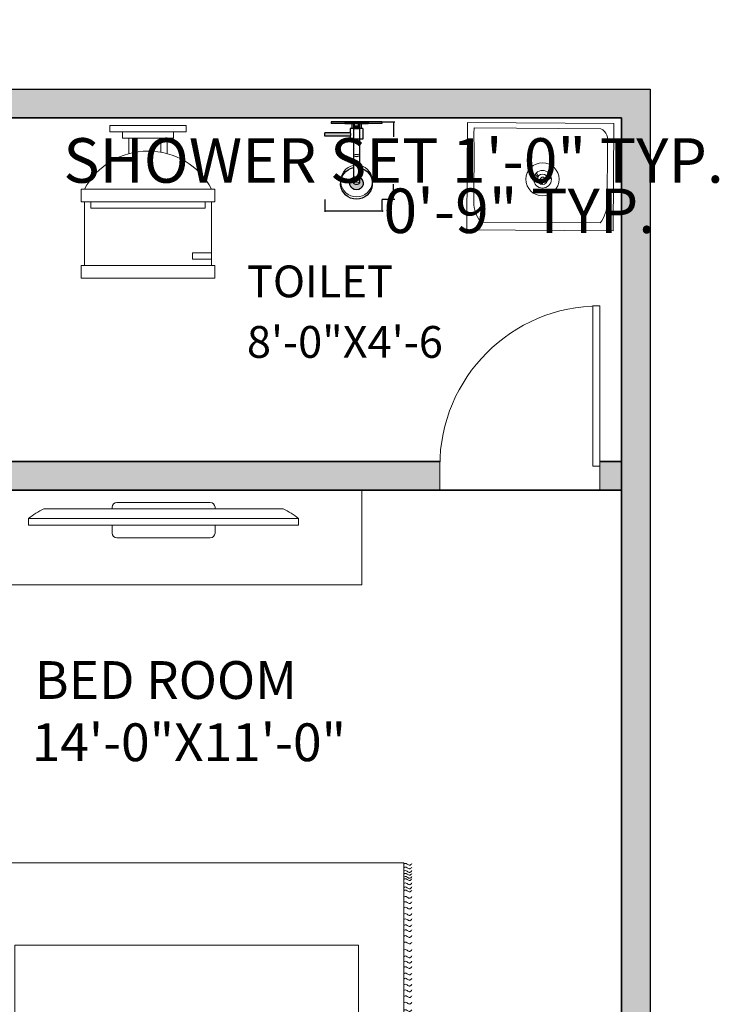
# Model space of a CAD drawing. Units: inches. Extents: x 0 to 4258, y 0 to 3769.
# Tile 28 of 30: x 3940 to 4050, y 3513 to 3668. Entities that reach past the tile are written whole.
import ezdxf

# ---------------------------------------------------------------- set-up
doc = ezdxf.new("R2010")
doc.units = ezdxf.units.IN
doc.header["$MEASUREMENT"] = 0
doc.layers.get('0').update_dxf_attribs({"color": 16})
for name, color, linetype, lineweight in [('A-ANNO-DIMS', 250, 'Continuous', 18), ('A-AREA-IDEN', 250, 'Continuous', 18), ('A-EQPM', 8, 'Continuous', 18), ('A-FLOR-FIXT', 250, 'Continuous', 18), ('A-WALL-PATT', 16, 'Continuous', 13), ('C-PROP', 150, 'Continuous', 25), ('doors', 250, 'Continuous', 18), ('furniture', 13, 'Continuous', 18), ('walls', 251, 'Continuous', 35)]:
    doc.layers.add(name, color=color, linetype=linetype, lineweight=lineweight)
doc.layers.add('PLUMBING FIXTURES', color=250, linetype='Continuous')
doc.styles.get("Standard").update_dxf_attribs({"font": 'arial.ttf'})
doc.dimstyles.get("Standard").update_dxf_attribs({"dimtxt": 7, "dimasz": 0.18, "dimexe": 0.18, "dimexo": 0.0625, "dimgap": 0.09, "dimtad": 0, "dimtih": 1, "dimtoh": 1, "dimzin": 0, "dimdsep": 46, "dimlunit": 3, "dimtxsty": 'Standard', "dimcen": 0.09, "dimadec": 0, "dimazin": 0, "dimtfac": 1, "dimtofl": 0, "dimtmove": 0, "dimatfit": 3, "dimfxl": 1, "dimtolj": 1, "dimtzin": 0, "dimarcsym": 0})

# ---------------------------------------------------------------- blocks, each defined once
blk = doc.blocks.new('PLASMA-LARGE')
at = {"layer": 'furniture'}
for p, q in [((-7.26, 0), (7.26, 0)), ((-18.61, -1), (18.61, -1)), ((-8, -1), (-8, -0.74)), ((8, -1), (8, -0.74)), ((-21, -2.5), (21, -2.5)), ((-21, -2.5), (-21, -3.5)), ((21, -2.5), (21, -3.5)), ((-21, -3.5), (21, -3.5)), ((-8, -3.5), (-8, -4.76)), ((8, -3.5), (8, -4.76)), ((-7.26, -5.5), (7.26, -5.5))]:
    blk.add_line(p, q, dxfattribs=at)
for centre, radius, start, end in [((-7.26, -0.74), 0.744, 90, 180), ((7.26, -0.74), 0.744, 0, 90), ((-13.97, -11.05), 11.07, 114.7602, 129.4175), ((13.97, -11.05), 11.07, 50.5825, 65.2398), ((-7.26, -4.76), 0.744, 180, 270), ((7.26, -4.76), 0.744, 270, 0)]:
    blk.add_arc(centre, radius, start, end, dxfattribs=at)
blk = doc.blocks.new('CARPET')
at = {"layer": 'furniture'}
for p, q in [((-51.53, -98.11), (-51.53, -55.12)), ((-51.53, -55.12), (-41.27, -55.12)), ((36, -55.12), (51.55, -55.12)), ((51.55, -55.12), (51.55, -98.11)), ((51.55, -98.11), (-51.53, -98.11))]:
    blk.add_line(p, q, dxfattribs=at)
for points, knots in [([(-53.37, -55.99), (-53.22, -55.8), (-52.9, -55.41), (-52.34, -55.8), (-51.89, -56.08), (-51.65, -55.91), (-51.53, -55.83)], [0, 0, 0, 0, 0.653278, 1.290138, 1.740457, 2.114451, 2.114451, 2.114451, 2.114451]), ([(-53.37, -57.26), (-53.22, -57.07), (-52.9, -56.67), (-52.34, -57.07), (-51.89, -57.35), (-51.65, -57.17), (-51.53, -57.1)], [0, 0, 0, 0, 0.653278, 1.290138, 1.740457, 2.114451, 2.114451, 2.114451, 2.114451]), ([(53.37, -55.99), (53.22, -55.8), (52.9, -55.41), (52.34, -55.8), (51.89, -56.08), (51.65, -55.91), (51.53, -55.83)], [0, 0, 0, 0, 0.653278, 1.290138, 1.740457, 2.114451, 2.114451, 2.114451, 2.114451]), ([(53.37, -57.26), (53.22, -57.07), (52.9, -56.67), (52.34, -57.07), (51.89, -57.35), (51.65, -57.17), (51.53, -57.1)], [0, 0, 0, 0, 0.653278, 1.290138, 1.740457, 2.114451, 2.114451, 2.114451, 2.114451]), ([(-53.37, -58.59), (-53.22, -58.4), (-52.9, -58.01), (-52.34, -58.4), (-51.89, -58.68), (-51.65, -58.5), (-51.53, -58.43)], [0, 0, 0, 0, 0.653278, 1.290138, 1.740457, 2.114451, 2.114451, 2.114451, 2.114451]), ([(-53.37, -59.78), (-53.22, -59.58), (-52.9, -59.19), (-52.34, -59.58), (-51.89, -59.86), (-51.65, -59.69), (-51.53, -59.61)], [0, 0, 0, 0, 0.653278, 1.290138, 1.740457, 2.114451, 2.114451, 2.114451, 2.114451]), ([(53.37, -58.59), (53.22, -58.4), (52.9, -58.01), (52.34, -58.4), (51.89, -58.68), (51.65, -58.5), (51.53, -58.43)], [0, 0, 0, 0, 0.653278, 1.290138, 1.740457, 2.114451, 2.114451, 2.114451, 2.114451]), ([(53.37, -59.78), (53.22, -59.58), (52.9, -59.19), (52.34, -59.58), (51.89, -59.86), (51.65, -59.69), (51.53, -59.61)], [0, 0, 0, 0, 0.653278, 1.290138, 1.740457, 2.114451, 2.114451, 2.114451, 2.114451]), ([(-53.37, -61.22), (-53.22, -61.02), (-52.9, -60.63), (-52.34, -61.02), (-51.89, -61.3), (-51.65, -61.13), (-51.53, -61.05)], [0, 0, 0, 0, 0.653278, 1.290138, 1.740457, 2.114451, 2.114451, 2.114451, 2.114451]), ([(-53.37, -62.44), (-53.22, -62.25), (-52.9, -61.86), (-52.34, -62.25), (-51.89, -62.53), (-51.65, -62.36), (-51.53, -62.28)], [0, 0, 0, 0, 0.653278, 1.290138, 1.740457, 2.114451, 2.114451, 2.114451, 2.114451]), ([(53.37, -61.22), (53.22, -61.02), (52.9, -60.63), (52.34, -61.02), (51.89, -61.3), (51.65, -61.13), (51.53, -61.05)], [0, 0, 0, 0, 0.653278, 1.290138, 1.740457, 2.114451, 2.114451, 2.114451, 2.114451]), ([(53.37, -62.44), (53.22, -62.25), (52.9, -61.86), (52.34, -62.25), (51.89, -62.53), (51.65, -62.36), (51.53, -62.28)], [0, 0, 0, 0, 0.653278, 1.290138, 1.740457, 2.114451, 2.114451, 2.114451, 2.114451]), ([(-53.37, -63.63), (-53.22, -63.43), (-52.9, -63.04), (-52.34, -63.43), (-51.89, -63.72), (-51.65, -63.54), (-51.53, -63.46)], [0, 0, 0, 0, 0.653278, 1.290138, 1.740457, 2.114451, 2.114451, 2.114451, 2.114451]), ([(53.37, -63.63), (53.22, -63.43), (52.9, -63.04), (52.34, -63.43), (51.89, -63.72), (51.65, -63.54), (51.53, -63.46)], [0, 0, 0, 0, 0.653278, 1.290138, 1.740457, 2.114451, 2.114451, 2.114451, 2.114451]), ([(-53.37, -65.07), (-53.22, -64.87), (-52.9, -64.48), (-52.34, -64.87), (-51.89, -65.15), (-51.65, -64.98), (-51.53, -64.9)], [0, 0, 0, 0, 0.653278, 1.290138, 1.740457, 2.114451, 2.114451, 2.114451, 2.114451]), ([(-53.37, -66.76), (-53.22, -66.56), (-52.9, -66.17), (-52.34, -66.56), (-51.89, -66.84), (-51.65, -66.67), (-51.53, -66.59)], [0, 0, 0, 0, 0.653278, 1.290138, 1.740457, 2.114451, 2.114451, 2.114451, 2.114451]), ([(53.37, -65.07), (53.22, -64.87), (52.9, -64.48), (52.34, -64.87), (51.89, -65.15), (51.65, -64.98), (51.53, -64.9)], [0, 0, 0, 0, 0.653278, 1.290138, 1.740457, 2.114451, 2.114451, 2.114451, 2.114451]), ([(53.37, -66.76), (53.22, -66.56), (52.9, -66.17), (52.34, -66.56), (51.89, -66.84), (51.65, -66.67), (51.53, -66.59)], [0, 0, 0, 0, 0.653278, 1.290138, 1.740457, 2.114451, 2.114451, 2.114451, 2.114451]), ([(-53.37, -68.2), (-53.22, -68), (-52.9, -67.61), (-52.34, -68), (-51.89, -68.28), (-51.65, -68.11), (-51.53, -68.03)], [0, 0, 0, 0, 0.653278, 1.290138, 1.740457, 2.114451, 2.114451, 2.114451, 2.114451]), ([(53.37, -68.2), (53.22, -68), (52.9, -67.61), (52.34, -68), (51.89, -68.28), (51.65, -68.11), (51.53, -68.03)], [0, 0, 0, 0, 0.653278, 1.290138, 1.740457, 2.114451, 2.114451, 2.114451, 2.114451]), ([(-53.37, -69.53), (-53.22, -69.33), (-52.9, -68.94), (-52.34, -69.33), (-51.89, -69.61), (-51.65, -69.44), (-51.53, -69.36)], [0, 0, 0, 0, 0.653278, 1.290138, 1.740457, 2.114451, 2.114451, 2.114451, 2.114451]), ([(-53.37, -70.79), (-53.22, -70.6), (-52.9, -70.21), (-52.34, -70.6), (-51.89, -70.88), (-51.65, -70.7), (-51.53, -70.63)], [0, 0, 0, 0, 0.653278, 1.290138, 1.740457, 2.114451, 2.114451, 2.114451, 2.114451]), ([(53.37, -69.53), (53.22, -69.33), (52.9, -68.94), (52.34, -69.33), (51.89, -69.61), (51.65, -69.44), (51.53, -69.36)], [0, 0, 0, 0, 0.653278, 1.290138, 1.740457, 2.114451, 2.114451, 2.114451, 2.114451]), ([(53.37, -70.79), (53.22, -70.6), (52.9, -70.21), (52.34, -70.6), (51.89, -70.88), (51.65, -70.7), (51.53, -70.63)], [0, 0, 0, 0, 0.653278, 1.290138, 1.740457, 2.114451, 2.114451, 2.114451, 2.114451]), ([(-53.37, -72.12), (-53.22, -71.93), (-52.9, -71.54), (-52.34, -71.93), (-51.89, -72.21), (-51.65, -72.04), (-51.53, -71.96)], [0, 0, 0, 0, 0.653278, 1.290138, 1.740457, 2.114451, 2.114451, 2.114451, 2.114451]), ([(-53.37, -73.31), (-53.22, -73.11), (-52.9, -72.72), (-52.34, -73.11), (-51.89, -73.4), (-51.65, -73.22), (-51.53, -73.14)], [0, 0, 0, 0, 0.653278, 1.290138, 1.740457, 2.114451, 2.114451, 2.114451, 2.114451]), ([(53.37, -72.12), (53.22, -71.93), (52.9, -71.54), (52.34, -71.93), (51.89, -72.21), (51.65, -72.04), (51.53, -71.96)], [0, 0, 0, 0, 0.653278, 1.290138, 1.740457, 2.114451, 2.114451, 2.114451, 2.114451]), ([(53.37, -73.31), (53.22, -73.11), (52.9, -72.72), (52.34, -73.11), (51.89, -73.4), (51.65, -73.22), (51.53, -73.14)], [0, 0, 0, 0, 0.653278, 1.290138, 1.740457, 2.114451, 2.114451, 2.114451, 2.114451]), ([(-53.37, -74.75), (-53.22, -74.55), (-52.9, -74.16), (-52.34, -74.55), (-51.89, -74.83), (-51.65, -74.66), (-51.53, -74.58)], [0, 0, 0, 0, 0.653278, 1.290138, 1.740457, 2.114451, 2.114451, 2.114451, 2.114451]), ([(53.37, -74.75), (53.22, -74.55), (52.9, -74.16), (52.34, -74.55), (51.89, -74.83), (51.65, -74.66), (51.53, -74.58)], [0, 0, 0, 0, 0.653278, 1.290138, 1.740457, 2.114451, 2.114451, 2.114451, 2.114451]), ([(-53.37, -75.98), (-53.22, -75.78), (-52.9, -75.39), (-52.34, -75.78), (-51.89, -76.06), (-51.65, -75.89), (-51.53, -75.81)], [0, 0, 0, 0, 0.653278, 1.290138, 1.740457, 2.114451, 2.114451, 2.114451, 2.114451]), ([(-53.37, -77.16), (-53.22, -76.96), (-52.9, -76.57), (-52.34, -76.96), (-51.89, -77.25), (-51.65, -77.07), (-51.53, -76.99)], [0, 0, 0, 0, 0.653278, 1.290138, 1.740457, 2.114451, 2.114451, 2.114451, 2.114451]), ([(53.37, -75.98), (53.22, -75.78), (52.9, -75.39), (52.34, -75.78), (51.89, -76.06), (51.65, -75.89), (51.53, -75.81)], [0, 0, 0, 0, 0.653278, 1.290138, 1.740457, 2.114451, 2.114451, 2.114451, 2.114451]), ([(53.37, -77.16), (53.22, -76.96), (52.9, -76.57), (52.34, -76.96), (51.89, -77.25), (51.65, -77.07), (51.53, -76.99)], [0, 0, 0, 0, 0.653278, 1.290138, 1.740457, 2.114451, 2.114451, 2.114451, 2.114451]), ([(-53.37, -78.6), (-53.22, -78.4), (-52.9, -78.01), (-52.34, -78.4), (-51.89, -78.68), (-51.65, -78.51), (-51.53, -78.43)], [0, 0, 0, 0, 0.653278, 1.290138, 1.740457, 2.114451, 2.114451, 2.114451, 2.114451]), ([(53.37, -78.6), (53.22, -78.4), (52.9, -78.01), (52.34, -78.4), (51.89, -78.68), (51.65, -78.51), (51.53, -78.43)], [0, 0, 0, 0, 0.653278, 1.290138, 1.740457, 2.114451, 2.114451, 2.114451, 2.114451]), ([(-53.37, -80.29), (-53.22, -80.09), (-52.9, -79.7), (-52.34, -80.09), (-51.89, -80.37), (-51.65, -80.2), (-51.53, -80.12)], [0, 0, 0, 0, 0.653278, 1.290138, 1.740457, 2.114451, 2.114451, 2.114451, 2.114451]), ([(-53.37, -81.73), (-53.22, -81.53), (-52.9, -81.14), (-52.34, -81.53), (-51.89, -81.81), (-51.65, -81.64), (-51.53, -81.56)], [0, 0, 0, 0, 0.653278, 1.290138, 1.740457, 2.114451, 2.114451, 2.114451, 2.114451]), ([(53.37, -80.29), (53.22, -80.09), (52.9, -79.7), (52.34, -80.09), (51.89, -80.37), (51.65, -80.2), (51.53, -80.12)], [0, 0, 0, 0, 0.653278, 1.290138, 1.740457, 2.114451, 2.114451, 2.114451, 2.114451]), ([(53.37, -81.73), (53.22, -81.53), (52.9, -81.14), (52.34, -81.53), (51.89, -81.81), (51.65, -81.64), (51.53, -81.56)], [0, 0, 0, 0, 0.653278, 1.290138, 1.740457, 2.114451, 2.114451, 2.114451, 2.114451]), ([(-53.37, -83.06), (-53.22, -82.86), (-52.9, -82.47), (-52.34, -82.86), (-51.89, -83.14), (-51.65, -82.97), (-51.53, -82.89)], [0, 0, 0, 0, 0.653278, 1.290138, 1.740457, 2.114451, 2.114451, 2.114451, 2.114451]), ([(-53.37, -84.18), (-53.22, -83.99), (-52.9, -83.6), (-52.34, -83.99), (-51.89, -84.27), (-51.65, -84.09), (-51.53, -84.02)], [0, 0, 0, 0, 0.653278, 1.290138, 1.740457, 2.114451, 2.114451, 2.114451, 2.114451]), ([(53.37, -83.06), (53.22, -82.86), (52.9, -82.47), (52.34, -82.86), (51.89, -83.14), (51.65, -82.97), (51.53, -82.89)], [0, 0, 0, 0, 0.653278, 1.290138, 1.740457, 2.114451, 2.114451, 2.114451, 2.114451]), ([(53.37, -84.18), (53.22, -83.99), (52.9, -83.6), (52.34, -83.99), (51.89, -84.27), (51.65, -84.09), (51.53, -84.02)], [0, 0, 0, 0, 0.653278, 1.290138, 1.740457, 2.114451, 2.114451, 2.114451, 2.114451]), ([(-53.37, -85.51), (-53.22, -85.32), (-52.9, -84.93), (-52.34, -85.32), (-51.89, -85.6), (-51.65, -85.42), (-51.53, -85.35)], [0, 0, 0, 0, 0.653278, 1.290138, 1.740457, 2.114451, 2.114451, 2.114451, 2.114451]), ([(-53.37, -86.7), (-53.22, -86.5), (-52.9, -86.11), (-52.34, -86.5), (-51.89, -86.78), (-51.65, -86.61), (-51.53, -86.53)], [0, 0, 0, 0, 0.653278, 1.290138, 1.740457, 2.114451, 2.114451, 2.114451, 2.114451]), ([(53.37, -85.51), (53.22, -85.32), (52.9, -84.93), (52.34, -85.32), (51.89, -85.6), (51.65, -85.42), (51.53, -85.35)], [0, 0, 0, 0, 0.653278, 1.290138, 1.740457, 2.114451, 2.114451, 2.114451, 2.114451]), ([(53.37, -86.7), (53.22, -86.5), (52.9, -86.11), (52.34, -86.5), (51.89, -86.78), (51.65, -86.61), (51.53, -86.53)], [0, 0, 0, 0, 0.653278, 1.290138, 1.740457, 2.114451, 2.114451, 2.114451, 2.114451]), ([(-53.37, -88.14), (-53.22, -87.94), (-52.9, -87.55), (-52.34, -87.94), (-51.89, -88.22), (-51.65, -88.05), (-51.53, -87.97)], [0, 0, 0, 0, 0.653278, 1.290138, 1.740457, 2.114451, 2.114451, 2.114451, 2.114451]), ([(53.37, -88.14), (53.22, -87.94), (52.9, -87.55), (52.34, -87.94), (51.89, -88.22), (51.65, -88.05), (51.53, -87.97)], [0, 0, 0, 0, 0.653278, 1.290138, 1.740457, 2.114451, 2.114451, 2.114451, 2.114451]), ([(-53.37, -89.36), (-53.22, -89.17), (-52.9, -88.78), (-52.34, -89.17), (-51.89, -89.45), (-51.65, -89.28), (-51.53, -89.2)], [0, 0, 0, 0, 0.653278, 1.290138, 1.740457, 2.114451, 2.114451, 2.114451, 2.114451]), ([(-53.37, -90.55), (-53.22, -90.35), (-52.9, -89.96), (-52.34, -90.35), (-51.89, -90.64), (-51.65, -90.46), (-51.53, -90.38)], [0, 0, 0, 0, 0.653278, 1.290138, 1.740457, 2.114451, 2.114451, 2.114451, 2.114451]), ([(53.37, -89.36), (53.22, -89.17), (52.9, -88.78), (52.34, -89.17), (51.89, -89.45), (51.65, -89.28), (51.53, -89.2)], [0, 0, 0, 0, 0.653278, 1.290138, 1.740457, 2.114451, 2.114451, 2.114451, 2.114451]), ([(53.37, -90.55), (53.22, -90.35), (52.9, -89.96), (52.34, -90.35), (51.9, -90.63), (51.66, -90.47), (51.55, -90.4)], [0, 0, 0, 0, 0.653278, 1.290138, 1.740457, 2.0926, 2.0926, 2.0926, 2.0926]), ([(-53.37, -91.99), (-53.22, -91.79), (-52.9, -91.4), (-52.34, -91.79), (-51.89, -92.07), (-51.65, -91.9), (-51.53, -91.82)], [0, 0, 0, 0, 0.653278, 1.290138, 1.740457, 2.114451, 2.114451, 2.114451, 2.114451]), ([(-53.37, -92.69), (-53.22, -92.48), (-52.9, -92.08), (-52.35, -92.49), (-51.89, -92.77), (-51.65, -92.6), (-51.53, -92.52)], [0, 0, 0, 0, 0.663904, 1.307406, 1.757725, 2.131719, 2.131719, 2.131719, 2.131719]), ([(53.37, -91.99), (53.22, -91.79), (52.9, -91.4), (52.34, -91.79), (51.9, -92.07), (51.66, -91.91), (51.55, -91.83)], [0, 0, 0, 0, 0.653278, 1.290138, 1.740457, 2.0926, 2.0926, 2.0926, 2.0926]), ([(53.37, -92.69), (53.22, -92.49), (52.9, -92.09), (52.34, -92.49), (51.9, -92.77), (51.66, -92.61), (51.55, -92.53)], [0, 0, 0, 0, 0.656792, 1.295826, 1.746145, 2.098292, 2.098292, 2.098292, 2.098292]), ([(-53.37, -93.61), (-53.22, -93.42), (-52.9, -93.03), (-52.34, -93.42), (-51.89, -93.7), (-51.65, -93.52), (-51.53, -93.45)], [0, 0, 0, 0, 0.653278, 1.290138, 1.740457, 2.114451, 2.114451, 2.114451, 2.114451]), ([(-53.37, -94.55), (-53.22, -94.35), (-52.9, -93.96), (-52.34, -94.35), (-51.89, -94.63), (-51.65, -94.46), (-51.53, -94.38)], [0, 0, 0, 0, 0.653278, 1.290138, 1.740457, 2.114451, 2.114451, 2.114451, 2.114451]), ([(-53.37, -95.05), (-53.22, -94.85), (-52.9, -94.46), (-52.34, -94.85), (-51.89, -95.14), (-51.65, -94.96), (-51.53, -94.88)], [0, 0, 0, 0, 0.653278, 1.290138, 1.740457, 2.114451, 2.114451, 2.114451, 2.114451]), ([(53.37, -93.66), (53.22, -93.46), (52.9, -93.07), (52.34, -93.46), (51.9, -93.74), (51.66, -93.58), (51.55, -93.5)], [0, 0, 0, 0, 0.653278, 1.290138, 1.740457, 2.0926, 2.0926, 2.0926, 2.0926]), ([(53.37, -94.59), (53.22, -94.4), (52.9, -94.01), (52.34, -94.4), (51.9, -94.68), (51.66, -94.51), (51.55, -94.44)], [0, 0, 0, 0, 0.653278, 1.290138, 1.740457, 2.0926, 2.0926, 2.0926, 2.0926]), ([(53.37, -95.1), (53.22, -94.9), (52.9, -94.51), (52.34, -94.9), (51.9, -95.18), (51.66, -95.02), (51.55, -94.94)], [0, 0, 0, 0, 0.653278, 1.290138, 1.740457, 2.0926, 2.0926, 2.0926, 2.0926]), ([(-53.37, -95.73), (-53.22, -95.54), (-52.9, -95.15), (-52.34, -95.54), (-51.89, -95.82), (-51.65, -95.65), (-51.53, -95.57)], [0, 0, 0, 0, 0.653278, 1.290138, 1.740457, 2.114451, 2.114451, 2.114451, 2.114451]), ([(-53.37, -96.38), (-53.22, -96.18), (-52.9, -95.79), (-52.34, -96.18), (-51.89, -96.47), (-51.65, -96.29), (-51.53, -96.21)], [0, 0, 0, 0, 0.653278, 1.290138, 1.740457, 2.114451, 2.114451, 2.114451, 2.114451]), ([(-53.37, -97.17), (-53.22, -96.98), (-52.9, -96.59), (-52.34, -96.98), (-51.89, -97.26), (-51.65, -97.08), (-51.53, -97.01)], [0, 0, 0, 0, 0.653278, 1.290138, 1.740457, 2.114451, 2.114451, 2.114451, 2.114451]), ([(53.37, -95.78), (53.22, -95.58), (52.9, -95.19), (52.34, -95.58), (51.89, -95.86), (51.65, -95.69), (51.53, -95.61)], [0, 0, 0, 0, 0.653278, 1.290138, 1.740457, 2.114451, 2.114451, 2.114451, 2.114451]), ([(53.37, -96.43), (53.22, -96.23), (52.9, -95.84), (52.34, -96.23), (51.89, -96.51), (51.65, -96.34), (51.53, -96.26)], [0, 0, 0, 0, 0.653278, 1.290138, 1.740457, 2.114451, 2.114451, 2.114451, 2.114451]), ([(53.37, -97.22), (53.22, -97.02), (52.9, -96.63), (52.34, -97.02), (51.89, -97.3), (51.65, -97.13), (51.53, -97.05)], [0, 0, 0, 0, 0.653278, 1.290138, 1.740457, 2.114451, 2.114451, 2.114451, 2.114451]), ([(-53.37, -97.99), (-53.22, -97.79), (-52.9, -97.4), (-52.34, -97.79), (-51.89, -98.08), (-51.65, -97.9), (-51.53, -97.82)], [0, 0, 0, 0, 0.653278, 1.290138, 1.740457, 2.114451, 2.114451, 2.114451, 2.114451]), ([(53.37, -97.99), (53.22, -97.79), (52.9, -97.4), (52.34, -97.79), (51.89, -98.08), (51.65, -97.9), (51.53, -97.82)], [0, 0, 0, 0, 0.653278, 1.290138, 1.740457, 2.114451, 2.114451, 2.114451, 2.114451])]:
    blk.add_open_spline(points, degree=3, knots=knots, dxfattribs=at)
blk = doc.blocks.new('A$C58D270C6')
at = {"layer": 'furniture'}
for p, q in [((9.09, 124.13), (9.09, 108.87)), ((1.46, 116.5), (16.73, 116.5)), ((14.97, 94.84), (24.62, 107.92)), ((24.62, 94.93), (24.62, 107.92)), ((42.08, 108), (42.08, 36)), ((14.97, 94.93), (24.62, 94.93)), ((14.97, 94.84), (14.97, 36)), ((16.22, 94.93), (16.22, 36)), ((9.25, 36), (9.25, 20.74)), ((1.62, 28.37), (16.88, 28.37))]:
    blk.add_line(p, q, dxfattribs=at)
for points in [[(18.5, 108), (18.34, 124.13), (-0.16, 124.13), (0, 108)], [(0, 108), (77.91, 108), (77.91, 36), (0, 36)], [(4.09, 94.93), (14.97, 94.93), (14.97, 73.83), (4.09, 73.83)], [(4.09, 65.23), (14.97, 65.23), (14.97, 44.13), (4.09, 44.13)], [(18.65, 19.87), (18.5, 36), (0, 36), (0.16, 19.87)]]:
    blk.add_lwpolyline(points, close=True, dxfattribs=at)
for centre in [(9.09, 116.5), (9.25, 28.37)]:
    blk.add_circle(centre, 5.95, dxfattribs=at)
at = {"layer": 'furniture', "xscale": 0.9312884925094044, "yscale": 0.9312884925094044, "zscale": 0.9312884925094044, "rotation": 90}
blk.add_blockref('CARPET', (3.79, 74.47), dxfattribs=at)
blk = doc.blocks.new('*U18')
for p, q in [((-10, 22), (-10, 12)), ((10, 12), (10, 22)), ((-10, 21), (-7, 21)), ((-7, 21), (-7, 20)), ((-7, 20), (-10, 20)), ((9, 13), (-9, 13)), ((-9, 13), (-9, 12)), ((9, 12), (9, 13)), ((10.5, 12), (-10.5, 12)), ((-10.5, 10), (-10.5, 12)), ((10.5, 12), (10.5, 10)), ((10.5, 10), (-10.5, 10)), ((-3, 4.4065), (-3, 2)), ((-2, 2), (-2, 4.1658)), ((2, 4.1658), (2, 2)), ((3, 2), (3, 4.4065)), ((4, 2), (-4, 2)), ((-4, 2), (-4, 1)), ((4, 1), (4, 2))]:
    blk.add_line(p, q)
for points in [[(10.5, 22), (10.5, 24), (-10.5, 24), (-10.5, 22)], [(6, 0), (6, 1), (-6, 1), (-6, 0)]]:
    blk.add_lwpolyline(points, close=True)
blk.add_arc((0, 15.3333), 11.3333, 208.0725, 331.9275)
blk = doc.blocks.new('*U23')
for p, q in [((0, 0), (0, -6)), ((40, 0), (40, -6))]:
    blk.add_line(p, q)
blk.add_lwpolyline([(0, 0), (0, 40), (1.75, 40), (1.75, 0)], close=True)
blk.add_arc((0, 0), 40, 0, 90)
blk = doc.blocks.new('BASIN-RECTANGULAR')
for p, q in [((0.01, 1.29), (0.11, 17)), ((0.11, 17), (23.11, 16.85)), ((1.16, 16.16), (21.05, 16.03)), ((23.11, 16.85), (23, 0)), ((1.14, 13.79), (1.08, 4.5)), ((22.11, 13.65), (22.05, 4.36)), ((11.13, 8.4), (10.74, 8.87)), ((11.26, 8.61), (10.89, 9.05)), ((11.75, 7.78), (11.7, 7.3)), ((11.88, 7.27), (11.94, 7.76)), ((12.59, 8.3), (13.23, 8.41)), ((12.71, 8.08), (13.27, 8.19)), ((0, 0.15), (0.01, 1.29)), ((23, 0), (0, 0.15)), ((2.14, 1.35), (20.95, 1.23))]:
    blk.add_line(p, q)
for radius in [2.61, 1.39, 0.816, 0.338]:
    blk.add_circle((11.89, 8.09), radius)
for centre, radius, start, end in [((10.4, 14.91), 9.33, 172.3124, 186.9318), ((20.1, 14.18), 2.08, 345.2338, 62.9258), ((6.48, 4.56), 5.4, 180.6949, 216.4918), ((16.65, 4.5), 5.4, 322.7525, 358.5493)]:
    blk.add_arc(centre, radius, start, end)
blk = doc.blocks.new('O.H SHOWER-PL')
at = {"layer": 'PLUMBING FIXTURES'}
for points in [[(-1.84, 0), (-1.84, -0.25), (1.84, -0.25), (1.84, 0)], [(0.46, -8.72), (0.46, -9.67, -0.422337), (-0.46, -9.67), (-0.46, -8.72, 4.325472)]]:
    blk.add_hatch(color=256, dxfattribs=at).paths.add_polyline_path(points)
for p, q in [((-1.84, 0), (-1.84, -0.25)), ((1.84, 0), (-1.84, 0)), ((1.84, 0), (1.84, -0.25)), ((1.84, -0.25), (-1.84, -0.25)), ((-0.46, -0.25), (-0.46, -9.67)), ((0.46, -0.25), (0.46, -9.67))]:
    blk.add_line(p, q, dxfattribs=at)
for centre, radius, start, end in [((0, -4.48), 1.03, 243.53, 296.47), ((0, -9.67), 2.5, 100.61, 79.39), ((0, -9.67), 1.05, 116.0349, 63.9652), ((0, -9.22), 0.643, 224.2078, 315.7922)]:
    blk.add_arc(centre, radius, start, end, dxfattribs=at)
blk = doc.blocks.new('DIVERTER-PL')
at = {"layer": 'PLUMBING FIXTURES'}
for points in [[(4, 0), (-4, 0), (-4, -0.25), (4, -0.25)], [(0.38, -1.14), (0.38, -0.7), (-0.37, -0.7), (-0.37, -1.14)], [(1, -1.75, 0.30818), (1, -2.25), (5, -2.25), (5, -1.75)]]:
    blk.add_hatch(color=256, dxfattribs=at).paths.add_polyline_path(points)
for p, q in [((-4, 0), (-4, -0.25)), ((-4, 0), (4, 0)), ((4, 0), (4, -0.25)), ((-4, -0.25), (4, -0.25)), ((-4, -0.25), (4, -0.25)), ((-1, -1.05), (-0.37, -1.05)), ((-1, -1.05), (-1, -2.75)), ((-0.75, -0.25), (-0.75, -1.05)), ((-0.37, -0.7), (0.38, -0.7)), ((-0.37, -0.7), (-0.37, -1.14)), ((-0.37, -1.14), (0.38, -1.14)), ((-0.32, -0.7), (-0.32, -0.25)), ((0.32, -0.7), (0.32, -0.25)), ((0.38, -0.7), (0.38, -1.14)), ((0.38, -1.05), (1, -1.05)), ((0.75, -0.25), (0.75, -1.05)), ((1, -1.05), (1, -1.75)), ((-1, -2.75), (1, -2.75)), ((1, -2.25), (1, -2.75))]:
    blk.add_line(p, q, dxfattribs=at)
at = {"layer": 'PLUMBING FIXTURES', "ltscale": 12}
for p, q in [((1, -1.75), (5, -1.75)), ((1, -2.25), (5, -2.25)), ((5, -2.25), (5, -1.75))]:
    blk.add_line(p, q, dxfattribs=at)
at = {"layer": 'PLUMBING FIXTURES'}
blk.add_arc((1.37, -2), 0.444, 145.7435, 214.2565, dxfattribs=at)
blk = doc.blocks.new('A$C7F153053')
at = {"layer": 'PLUMBING FIXTURES', "xscale": -1, "rotation": 270}
for name in ['DIVERTER-PL', 'O.H SHOWER-PL']:
    blk.add_blockref(name, (12.17, 4), dxfattribs=at)
blk = doc.blocks.new('SHOWER-WALL-SET')
blk.add_hatch(color=256).paths.add_polyline_path([(5.46, 1.56), (5.46, 2.5, 0.422337), (4.54, 2.5), (4.54, 1.56, -4.325472)])
blk.add_hatch(color=256).paths.add_polyline_path([(5.46, 1.56), (5.46, 2.5, 0.422337), (4.54, 2.5), (4.54, 1.56, -4.325472)])
blk.add_hatch(color=256).paths.add_polyline_path([(5.46, 1.56), (5.46, 2.5, 0.422337), (4.54, 2.5), (4.54, 1.56, -4.325472)])
blk.add_hatch(color=256).paths.add_polyline_path([(5.46, 1.56), (5.46, 2.5, 0.422337), (4.54, 2.5), (4.54, 1.56, -4.325472)])
blk.add_hatch(color=256).paths.add_polyline_path([(5.46, 1.56), (5.46, 2.5, 0.422337), (4.54, 2.5), (4.54, 1.56, -4.325472)])
blk.add_hatch(color=256).paths.add_polyline_path([(5.46, 1.56), (5.46, 2.5, 0.422337), (4.54, 2.5), (4.54, 1.56, -4.325472)])
blk.add_hatch(color=256).paths.add_polyline_path([(5.46, 1.56), (5.46, 2.5, 0.422337), (4.54, 2.5), (4.54, 1.56, -4.325472)])
blk.add_hatch(color=256).paths.add_polyline_path([(5.46, 1.56), (5.46, 2.5, 0.422337), (4.54, 2.5), (4.54, 1.56, -4.325472)])
blk.add_hatch(color=256).paths.add_polyline_path([(5.46, 1.56), (5.46, 2.5, 0.422337), (4.54, 2.5), (4.54, 1.56, -4.325472)])
blk.add_hatch(color=256).paths.add_polyline_path([(5.46, 1.56), (5.46, 2.5, 0.422337), (4.54, 2.5), (4.54, 1.56, -4.325472)])
blk.add_hatch(color=256).paths.add_polyline_path([(5.46, 1.56), (5.46, 2.5, 0.422337), (4.54, 2.5), (4.54, 1.56, -4.325472)])
blk.add_hatch(color=256).paths.add_polyline_path([(5.46, 1.56), (5.46, 2.5, 0.422337), (4.54, 2.5), (4.54, 1.56, -4.325472)])
blk.add_hatch(color=256).paths.add_polyline_path([(5.46, 1.56), (5.46, 2.5, 0.422337), (4.54, 2.5), (4.54, 1.56, -4.325472)])
blk.add_hatch(color=256).paths.add_polyline_path([(5.46, 1.56), (5.46, 2.5, 0.422337), (4.54, 2.5), (4.54, 1.56, -4.325472)])
blk.add_hatch(color=256).paths.add_polyline_path([(5.46, 1.56), (5.46, 2.5, 0.422337), (4.54, 2.5), (4.54, 1.56, -4.325472)])
blk.add_hatch(color=256).paths.add_polyline_path([(5.46, 1.56), (5.46, 2.5, 0.422337), (4.54, 2.5), (4.54, 1.56, -4.325472)])
blk.add_hatch(color=256).paths.add_polyline_path([(5.46, 1.56), (5.46, 2.5, 0.422337), (4.54, 2.5), (4.54, 1.56, -4.325472)])
blk.add_hatch(color=256).paths.add_polyline_path([(5.46, 1.56), (5.46, 2.5, 0.422337), (4.54, 2.5), (4.54, 1.56, -4.325472)])
blk.add_hatch(color=256).paths.add_polyline_path([(5.46, 1.56), (5.46, 2.5, 0.422337), (4.54, 2.5), (4.54, 1.56, -4.325472)])
blk.add_hatch(color=256).paths.add_polyline_path([(5.46, 1.56), (5.46, 2.5, 0.422337), (4.54, 2.5), (4.54, 1.56, -4.325472)])
blk.add_hatch(color=256).paths.add_polyline_path([(5.46, 1.56), (5.46, 2.5, 0.422337), (4.54, 2.5), (4.54, 1.56, -4.325472)])
blk.add_hatch(color=256).paths.add_polyline_path([(5.46, 1.56), (5.46, 2.5, 0.422337), (4.54, 2.5), (4.54, 1.56, -4.325472)])
blk.add_hatch(color=256).paths.add_polyline_path([(5.46, 1.56), (5.46, 2.5, 0.422337), (4.54, 2.5), (4.54, 1.56, -4.325472)])
blk.add_hatch(color=256).paths.add_polyline_path([(5.46, 1.56), (5.46, 2.5, 0.422337), (4.54, 2.5), (4.54, 1.56, -4.325472)])
blk.add_hatch(color=256).paths.add_polyline_path([(5.46, 1.56), (5.46, 2.5, 0.422337), (4.54, 2.5), (4.54, 1.56, -4.325472)])
blk.add_hatch(color=256).paths.add_polyline_path([(5.46, 1.56), (5.46, 2.5, 0.422337), (4.54, 2.5), (4.54, 1.56, -4.325472)])
blk.add_hatch(color=256).paths.add_polyline_path([(5.46, 1.56), (5.46, 2.5, 0.422337), (4.54, 2.5), (4.54, 1.56, -4.325472)])
blk.add_hatch(color=256).paths.add_polyline_path([(5.46, 1.56), (5.46, 2.5, 0.422337), (4.54, 2.5), (4.54, 1.56, -4.325472)])
blk.add_hatch(color=256).paths.add_polyline_path([(5.46, 1.56), (5.46, 2.5, 0.422337), (4.54, 2.5), (4.54, 1.56, -4.325472)])
blk.add_hatch(color=256).paths.add_polyline_path([(5.46, 1.56), (5.46, 2.5, 0.422337), (4.54, 2.5), (4.54, 1.56, -4.325472)])
blk.add_hatch(color=256).paths.add_polyline_path([(5.46, 1.56), (5.46, 2.5, 0.422337), (4.54, 2.5), (4.54, 1.56, -4.325472)])
blk.add_hatch(color=256).paths.add_polyline_path([(5.46, 1.56), (5.46, 2.5, 0.422337), (4.54, 2.5), (4.54, 1.56, -4.325472)])
blk.add_hatch(color=256).paths.add_polyline_path([(5.46, 1.56), (5.46, 2.5, 0.422337), (4.54, 2.5), (4.54, 1.56, -4.325472)])
blk.add_hatch(color=256).paths.add_polyline_path([(5.46, 1.56), (5.46, 2.5, 0.422337), (4.54, 2.5), (4.54, 1.56, -4.325472)])
blk.add_hatch(color=256).paths.add_polyline_path([(5.46, 1.56), (5.46, 2.5, 0.422337), (4.54, 2.5), (4.54, 1.56, -4.325472)])
blk.add_hatch(color=256).paths.add_polyline_path([(5.46, 1.56), (5.46, 2.5, 0.422337), (4.54, 2.5), (4.54, 1.56, -4.325472)])
blk.add_hatch(color=256).paths.add_polyline_path([(5.46, 1.56), (5.46, 2.5, 0.422337), (4.54, 2.5), (4.54, 1.56, -4.325472)])
blk.add_hatch(color=256).paths.add_polyline_path([(5.46, 1.56), (5.46, 2.5, 0.422337), (4.54, 2.5), (4.54, 1.56, -4.325472)])
for p, q in [((4.54, 11.92), (4.54, 2.5)), ((4.54, 11.92), (4.54, 2.5)), ((4.54, 11.92), (4.54, 2.5)), ((4.54, 11.92), (4.54, 2.5)), ((4.54, 11.92), (4.54, 2.5)), ((4.54, 11.92), (4.54, 2.5)), ((4.54, 11.92), (4.54, 2.5)), ((4.54, 11.92), (4.54, 2.5)), ((4.54, 11.92), (4.54, 2.5)), ((4.54, 11.92), (4.54, 2.5)), ((4.54, 11.92), (4.54, 2.5)), ((4.54, 11.92), (4.54, 2.5)), ((4.54, 11.92), (4.54, 2.5)), ((4.54, 11.92), (4.54, 2.5)), ((4.54, 11.92), (4.54, 2.5)), ((4.54, 11.92), (4.54, 2.5)), ((4.54, 11.92), (4.54, 2.5)), ((4.54, 11.92), (4.54, 2.5)), ((4.54, 11.92), (4.54, 2.5)), ((4.54, 11.92), (4.54, 2.5)), ((4.54, 11.92), (4.54, 2.5)), ((4.54, 11.92), (4.54, 2.5)), ((4.54, 11.92), (4.54, 2.5)), ((4.54, 11.92), (4.54, 2.5)), ((4.54, 11.92), (4.54, 2.5)), ((4.54, 11.92), (4.54, 2.5)), ((4.54, 11.92), (4.54, 2.5)), ((4.54, 11.92), (4.54, 2.5)), ((4.54, 11.92), (4.54, 2.5)), ((4.54, 11.92), (4.54, 2.5)), ((4.54, 11.92), (4.54, 2.5)), ((4.54, 11.92), (4.54, 2.5)), ((4.54, 11.92), (4.54, 2.5)), ((4.54, 11.92), (4.54, 2.5)), ((4.54, 11.92), (4.54, 2.5)), ((4.54, 11.92), (4.54, 2.5)), ((4.54, 11.92), (4.54, 2.5)), ((4.54, 11.92), (4.54, 2.5)), ((5.46, 11.92), (5.46, 2.5)), ((5.46, 11.92), (5.46, 2.5)), ((5.46, 11.92), (5.46, 2.5)), ((5.46, 11.92), (5.46, 2.5)), ((5.46, 11.92), (5.46, 2.5)), ((5.46, 11.92), (5.46, 2.5)), ((5.46, 11.92), (5.46, 2.5)), ((5.46, 11.92), (5.46, 2.5)), ((5.46, 11.92), (5.46, 2.5)), ((5.46, 11.92), (5.46, 2.5)), ((5.46, 11.92), (5.46, 2.5)), ((5.46, 11.92), (5.46, 2.5)), ((5.46, 11.92), (5.46, 2.5)), ((5.46, 11.92), (5.46, 2.5)), ((5.46, 11.92), (5.46, 2.5)), ((5.46, 11.92), (5.46, 2.5)), ((5.46, 11.92), (5.46, 2.5)), ((5.46, 11.92), (5.46, 2.5)), ((5.46, 11.92), (5.46, 2.5)), ((5.46, 11.92), (5.46, 2.5)), ((5.46, 11.92), (5.46, 2.5)), ((5.46, 11.92), (5.46, 2.5)), ((5.46, 11.92), (5.46, 2.5)), ((5.46, 11.92), (5.46, 2.5)), ((5.46, 11.92), (5.46, 2.5)), ((5.46, 11.92), (5.46, 2.5)), ((5.46, 11.92), (5.46, 2.5)), ((5.46, 11.92), (5.46, 2.5)), ((5.46, 11.92), (5.46, 2.5)), ((5.46, 11.92), (5.46, 2.5)), ((5.46, 11.92), (5.46, 2.5)), ((5.46, 11.92), (5.46, 2.5)), ((5.46, 11.92), (5.46, 2.5)), ((5.46, 11.92), (5.46, 2.5)), ((5.46, 11.92), (5.46, 2.5)), ((5.46, 11.92), (5.46, 2.5)), ((5.46, 11.92), (5.46, 2.5)), ((5.46, 11.92), (5.46, 2.5))]:
    blk.add_line(p, q)
for centre, radius, start, end in [((5.01, 8.04), 1.03, 243.53, 296.47), ((5.01, 8.04), 1.03, 243.53, 296.47), ((5.01, 8.04), 1.03, 243.53, 296.47), ((5.01, 8.04), 1.03, 243.53, 296.47), ((5.01, 8.04), 1.03, 243.53, 296.47), ((5.01, 8.04), 1.03, 243.53, 296.47), ((5.01, 8.04), 1.03, 243.53, 296.47), ((5.01, 8.04), 1.03, 243.53, 296.47), ((5.01, 8.04), 1.03, 243.53, 296.47), ((5.01, 8.04), 1.03, 243.53, 296.47), ((5.01, 8.04), 1.03, 243.53, 296.47), ((5.01, 8.04), 1.03, 243.53, 296.47), ((5.01, 8.04), 1.03, 243.53, 296.47), ((5.01, 8.04), 1.03, 243.53, 296.47), ((5.01, 8.04), 1.03, 243.53, 296.47), ((5.01, 8.04), 1.03, 243.53, 296.47), ((5.01, 8.04), 1.03, 243.53, 296.47), ((5.01, 8.04), 1.03, 243.53, 296.47), ((5.01, 8.04), 1.03, 243.53, 296.47), ((5.01, 8.04), 1.03, 243.53, 296.47), ((5.01, 8.04), 1.03, 243.53, 296.47), ((5.01, 8.04), 1.03, 243.53, 296.47), ((5.01, 8.04), 1.03, 243.53, 296.47), ((5.01, 8.04), 1.03, 243.53, 296.47), ((5.01, 8.04), 1.03, 243.53, 296.47), ((5.01, 8.04), 1.03, 243.53, 296.47), ((5.01, 8.04), 1.03, 243.53, 296.47), ((5.01, 8.04), 1.03, 243.53, 296.47), ((5.01, 8.04), 1.03, 243.53, 296.47), ((5.01, 8.04), 1.03, 243.53, 296.47), ((5.01, 8.04), 1.03, 243.53, 296.47), ((5.01, 8.04), 1.03, 243.53, 296.47), ((5.01, 8.04), 1.03, 243.53, 296.47), ((5.01, 8.04), 1.03, 243.53, 296.47), ((5.01, 8.04), 1.03, 243.53, 296.47), ((5.01, 8.04), 1.03, 243.53, 296.47), ((5.01, 8.04), 1.03, 243.53, 296.47), ((5.01, 8.04), 1.03, 243.53, 296.47), ((5.01, 2.85), 2.5, 100.61, 79.39), ((5.01, 2.85), 2.5, 100.61, 79.39), ((5.01, 2.85), 2.5, 100.61, 79.39), ((5.01, 2.85), 2.5, 100.61, 79.39), ((5.01, 2.85), 2.5, 100.61, 79.39), ((5.01, 2.85), 2.5, 100.61, 79.39), ((5.01, 2.85), 2.5, 100.61, 79.39), ((5.01, 2.85), 2.5, 100.61, 79.39), ((5.01, 2.85), 2.5, 100.61, 79.39), ((5.01, 2.85), 2.5, 100.61, 79.39), ((5.01, 2.85), 2.5, 100.61, 79.39), ((5.01, 2.85), 2.5, 100.61, 79.39), ((5.01, 2.85), 2.5, 100.61, 79.39), ((5.01, 2.85), 2.5, 100.61, 79.39), ((5.01, 2.85), 2.5, 100.61, 79.39), ((5.01, 2.85), 2.5, 100.61, 79.39), ((5.01, 2.85), 2.5, 100.61, 79.39), ((5.01, 2.85), 2.5, 100.61, 79.39), ((5.01, 2.85), 2.5, 100.61, 79.39), ((5.01, 2.85), 2.5, 100.61, 79.39), ((5.01, 2.85), 2.5, 100.61, 79.39), ((5.01, 2.85), 2.5, 100.61, 79.39), ((5.01, 2.85), 2.5, 100.61, 79.39), ((5.01, 2.85), 2.5, 100.61, 79.39), ((5.01, 2.85), 2.5, 100.61, 79.39), ((5.01, 2.85), 2.5, 100.61, 79.39), ((5.01, 2.85), 2.5, 100.61, 79.39), ((5.01, 2.85), 2.5, 100.61, 79.39), ((5.01, 2.85), 2.5, 100.61, 79.39), ((5.01, 2.85), 2.5, 100.61, 79.39), ((5.01, 2.85), 2.5, 100.61, 79.39), ((5.01, 2.85), 2.5, 100.61, 79.39), ((5.01, 2.85), 2.5, 100.61, 79.39), ((5.01, 2.85), 2.5, 100.61, 79.39), ((5.01, 2.85), 2.5, 100.61, 79.39), ((5.01, 2.85), 2.5, 100.61, 79.39), ((5.01, 2.85), 2.5, 100.61, 79.39), ((5.01, 2.85), 2.5, 100.61, 79.39), ((5, 2.5), 1.05, 296.0348, 243.9651), ((5, 2.5), 1.05, 296.0348, 243.9651), ((5, 2.5), 1.05, 296.0348, 243.9651), ((5, 2.5), 1.05, 296.0348, 243.9651), ((5, 2.5), 1.05, 296.0348, 243.9651), ((5, 2.5), 1.05, 296.0348, 243.9651), ((5, 2.5), 1.05, 296.0348, 243.9651), ((5, 2.5), 1.05, 296.0348, 243.9651), ((5, 2.5), 1.05, 296.0348, 243.9651), ((5, 2.5), 1.05, 296.0348, 243.9651), ((5, 2.5), 1.05, 296.0348, 243.9651), ((5, 2.5), 1.05, 296.0348, 243.9651), ((5, 2.5), 1.05, 296.0348, 243.9651), ((5, 2.5), 1.05, 296.0348, 243.9651), ((5, 2.5), 1.05, 296.0348, 243.9651), ((5, 2.5), 1.05, 296.0348, 243.9651), ((5, 2.5), 1.05, 296.0348, 243.9651), ((5, 2.5), 1.05, 296.0348, 243.9651), ((5, 2.5), 1.05, 296.0348, 243.9651), ((5, 2.5), 1.05, 296.0348, 243.9651), ((5, 2.5), 1.05, 296.0348, 243.9651), ((5, 2.5), 1.05, 296.0348, 243.9651), ((5, 2.5), 1.05, 296.0348, 243.9651), ((5, 2.5), 1.05, 296.0348, 243.9651), ((5, 2.5), 1.05, 296.0348, 243.9651), ((5, 2.5), 1.05, 296.0348, 243.9651), ((5, 2.5), 1.05, 296.0348, 243.9651), ((5, 2.5), 1.05, 296.0348, 243.9651), ((5, 2.5), 1.05, 296.0348, 243.9651), ((5, 2.5), 1.05, 296.0348, 243.9651), ((5, 2.5), 1.05, 296.0348, 243.9651), ((5, 2.5), 1.05, 296.0348, 243.9651), ((5, 2.5), 1.05, 296.0348, 243.9651), ((5, 2.5), 1.05, 296.0348, 243.9651), ((5, 2.5), 1.05, 296.0348, 243.9651), ((5, 2.5), 1.05, 296.0348, 243.9651), ((5, 2.5), 1.05, 296.0348, 243.9651), ((5, 2.5), 1.05, 296.0348, 243.9651), ((5, 2.05), 0.643, 44.2078, 135.7922), ((5, 2.05), 0.643, 44.2078, 135.7922), ((5, 2.05), 0.643, 44.2078, 135.7922), ((5, 2.05), 0.643, 44.2078, 135.7922), ((5, 2.05), 0.643, 44.2078, 135.7922), ((5, 2.05), 0.643, 44.2078, 135.7922), ((5, 2.05), 0.643, 44.2078, 135.7922), ((5, 2.05), 0.643, 44.2078, 135.7922), ((5, 2.05), 0.643, 44.2078, 135.7922), ((5, 2.05), 0.643, 44.2078, 135.7922), ((5, 2.05), 0.643, 44.2078, 135.7922), ((5, 2.05), 0.643, 44.2078, 135.7922), ((5, 2.05), 0.643, 44.2078, 135.7922), ((5, 2.05), 0.643, 44.2078, 135.7922), ((5, 2.05), 0.643, 44.2078, 135.7922), ((5, 2.05), 0.643, 44.2078, 135.7922), ((5, 2.05), 0.643, 44.2078, 135.7922), ((5, 2.05), 0.643, 44.2078, 135.7922), ((5, 2.05), 0.643, 44.2078, 135.7922), ((5, 2.05), 0.643, 44.2078, 135.7922), ((5, 2.05), 0.643, 44.2078, 135.7922), ((5, 2.05), 0.643, 44.2078, 135.7922), ((5, 2.05), 0.643, 44.2078, 135.7922), ((5, 2.05), 0.643, 44.2078, 135.7922), ((5, 2.05), 0.643, 44.2078, 135.7922), ((5, 2.05), 0.643, 44.2078, 135.7922), ((5, 2.05), 0.643, 44.2078, 135.7922), ((5, 2.05), 0.643, 44.2078, 135.7922), ((5, 2.05), 0.643, 44.2078, 135.7922), ((5, 2.05), 0.643, 44.2078, 135.7922), ((5, 2.05), 0.643, 44.2078, 135.7922), ((5, 2.05), 0.643, 44.2078, 135.7922), ((5, 2.05), 0.643, 44.2078, 135.7922), ((5, 2.05), 0.643, 44.2078, 135.7922), ((5, 2.05), 0.643, 44.2078, 135.7922), ((5, 2.05), 0.643, 44.2078, 135.7922), ((5, 2.05), 0.643, 44.2078, 135.7922), ((5, 2.05), 0.643, 44.2078, 135.7922)]:
    blk.add_arc(centre, radius, start, end)
at = {"ltscale": 35, "rotation": 89.99999999999999}
blk.add_blockref('A$C7F153053', (9, 0), dxfattribs=at)
blk = doc.blocks.new('TV-CONSOLE-CABINET')
for p, q in [((0, 0), (0, 64.44)), ((0, 64.44), (14.9, 64.44)), ((14.9, 0), (0, 0))]:
    blk.add_line(p, q)
blk = doc.blocks.new('*D60')
at = {"layer": 'A-ANNO-DIMS', "color": 0, "lineweight": -2, "transparency": 16777216}
for p, q in [((3996.71, 3651.69), (3998.66, 3651.69)), ((3998.48, 3651.51), (3998.48, 3649.32)), ((3998.48, 3639.71), (3998.48, 3641.9)), ((3996.71, 3639.53), (3998.66, 3639.53))]:
    blk.add_line(p, q, dxfattribs=at)
at = {"layer": 'A-ANNO-DIMS', "color": 0, "transparency": 16777216}
for points in [[(3998.45, 3651.51), (3998.51, 3651.51), (3998.48, 3651.69)], [(3998.45, 3639.71), (3998.51, 3639.71), (3998.48, 3639.53)]]:
    blk.add_solid(points, dxfattribs=at)
at = {"layer": 'Defpoints', "color": 0, "transparency": 16777216}
for p in [(3996.65, 3651.69), (3998.48, 3651.69), (3996.65, 3639.53)]:
    blk.add_point(p, dxfattribs=at)
at = {"layer": 'A-ANNO-DIMS', "color": 0, "transparency": 16777216, "insert": (3998.48, 3645.61), "char_height": 7, "attachment_point": 5}
blk.add_mtext('\\A1;SHOWER SET 1\'-0" TYP.', dxfattribs=at)
blk = doc.blocks.new('*D61')
at = {"layer": 'A-ANNO-DIMS', "color": 0, "lineweight": -2, "transparency": 16777216}
for p, q in [((3987.65, 3639.46), (3987.65, 3637.52)), ((3996.65, 3639.46), (3996.65, 3637.52)), ((3987.83, 3637.7), (3996.47, 3637.7)), ((3996.65, 3637.7), (3996.83, 3637.7))]:
    blk.add_line(p, q, dxfattribs=at)
at = {"layer": 'A-ANNO-DIMS', "color": 0, "transparency": 16777216}
for points in [[(3987.83, 3637.73), (3987.83, 3637.67), (3987.65, 3637.7)], [(3996.47, 3637.73), (3996.47, 3637.67), (3996.65, 3637.7)]]:
    blk.add_solid(points, dxfattribs=at)
at = {"layer": 'Defpoints', "color": 0, "transparency": 16777216}
for p in [(3987.65, 3639.53), (3996.65, 3639.53), (3996.65, 3637.7)]:
    blk.add_point(p, dxfattribs=at)
at = {"layer": 'A-ANNO-DIMS', "color": 0, "transparency": 16777216, "insert": (4018.25, 3637.7), "char_height": 7, "attachment_point": 5}
blk.add_mtext('\\A1;0\'-9" TYP.', dxfattribs=at)

msp = doc.modelspace()

# ---------------------------------------------------------------- hatches: boundary and pattern name
at = {"layer": 'A-WALL-PATT'}
h = msp.add_hatch(color=256, dxfattribs=at)
h.dxf.hatch_style = 1
h.paths.add_polyline_path([(3866.304, 3343.984), (3861.804, 3343.984), (3861.804, 3251.848), (3866.304, 3251.848)])
h.paths.add_polyline_path([(3881.946, 3330.642), (3866.304, 3330.642), (3866.304, 3326.142), (3881.946, 3326.142)])
h.paths.add_polyline_path([(4038.804, 3656.793), (3933.804, 3656.793), (3933.804, 3638.769), (3938.304, 3638.769), (3938.304, 3652.293), (4034.304, 3652.293), (4034.304, 3260.793), (4030.207, 3260.793), (4030.207, 3256.293), (4038.804, 3256.293)])
h = msp.add_hatch(color=256, dxfattribs=at)
h.dxf.hatch_style = 1
h.paths.add_polyline_path([(4005.754, 3597.57, -0.0071857), (4005.764, 3598.293), (3938.304, 3598.293), (3938.304, 3617.728), (3933.804, 3617.728), (3933.804, 3598.293), (3926.508, 3598.293), (3926.508, 3593.793), (4005.754, 3593.793)])
h = msp.add_hatch(color=256, dxfattribs=at)
h.dxf.hatch_style = 1
h.paths.add_polyline_path([(4030.944, 3598.293), (4030.89, 3593.793), (4034.304, 3593.793), (4034.304, 3598.293)])

# ---------------------------------------------------------------- linework, layer by layer
at = {"layer": 'C-PROP'}
for p, q in [((3678.804, 3656.793), (4038.804, 3656.793)), ((4038.804, 3656.793), (4038.804, 2936.793))]:
    msp.add_line(p, q, dxfattribs=at)
at = {"layer": 'walls'}
for p, q in [((3938.304, 3652.293), (4034.304, 3652.293)), ((4034.304, 3652.293), (4034.304, 3260.793)), ((3938.304, 3598.293), (4005.764, 3598.293)), ((4030.944, 3598.293), (4034.304, 3598.293)), ((4032.27, 3598.293), (4034.304, 3598.293)), ((3866.304, 3593.793), (4034.304, 3593.793))]:
    msp.add_line(p, q, dxfattribs=at)

# ---------------------------------------------------------------- block references
at = {"layer": 'A-EQPM', "xscale": 1.011294184530666, "yscale": 1.011294184530666, "zscale": 1.011294184530666}
msp.add_blockref('PLASMA-LARGE', (3962.312, 3591.843), dxfattribs=at)
at = {"layer": 'A-FLOR-FIXT'}
for name, p in [('SHOWER-WALL-SET', (3987.65, 3639.525)), ('BASIN-RECTANGULAR', (4010.016, 3634.557))]:
    msp.add_blockref(name, p, dxfattribs=at)
at = {"layer": 'A-FLOR-FIXT', "rotation": 180}
msp.add_blockref('*U18', (3959.871, 3651.091), dxfattribs=at)
at = {"layer": 'doors', "xscale": -0.6294121846440242, "yscale": 0.6294121846440242, "zscale": 0.6294121846440242}
msp.add_blockref('*U23', (4030.931, 3597.57), dxfattribs=at)
at = {"layer": 'furniture', "rotation": 89.9999999999983}
msp.add_blockref('TV-CONSOLE-CABINET', (3993.494, 3578.897), dxfattribs=at)
at = {"layer": 'furniture', "xscale": 0.7500000390647866, "yscale": 0.7500000390647866, "zscale": 0.7500000390647866, "rotation": 90}
msp.add_blockref('A$C58D270C6', (4019.941, 3463.822), dxfattribs=at)

# ---------------------------------------------------------------- texts
at = {"layer": 'A-AREA-IDEN'}
for s, height, p in [('TOILET', 5, (3975.42, 3624.099)), ('8\'-0"X4\'-6', 5, (3975.42, 3614.584)), ('BED ROOM', 5.939, (3942.067, 3560.963)), ('14\'-0"X11\'-0"', 5.93898, (3941.57, 3551.181))]:
    msp.add_text(s, height=height, dxfattribs=at).set_placement(p)

# ---------------------------------------------------------------- dimensions: what is measured, and where the dimension line sits
at = {"layer": 'A-ANNO-DIMS'}
dim = msp.add_linear_dim(base=(3998.476, 3651.693), p1=(3996.65, 3639.525), p2=(3996.65, 3651.693), angle=90, text='SHOWER SET <> TYP.', dimstyle='Standard', override={"dimdec": 1, "dimlfac": 1, "dimrnd": 0, "dimzin": 1, "dimdsep": 46, "dimlunit": 4, "dimfrac": 2}, dxfattribs=at)
dim.commit()
dim.dimension.update_dxf_attribs({"geometry": '*D60', "text_midpoint": (3998.476, 3645.609)})
dim = msp.add_linear_dim(base=(3996.65, 3637.7), p1=(3987.65, 3639.525), p2=(3996.65, 3639.525), text='<> TYP.', dimstyle='Standard', override={"dimdec": 1, "dimlfac": 1, "dimrnd": 0, "dimzin": 1, "dimdsep": 46, "dimlunit": 4, "dimfrac": 2}, dxfattribs=at)
dim.commit()
dim.dimension.update_dxf_attribs({"geometry": '*D61', "text_midpoint": (4018.255, 3637.7)})

doc.saveas('drawing.dxf')
